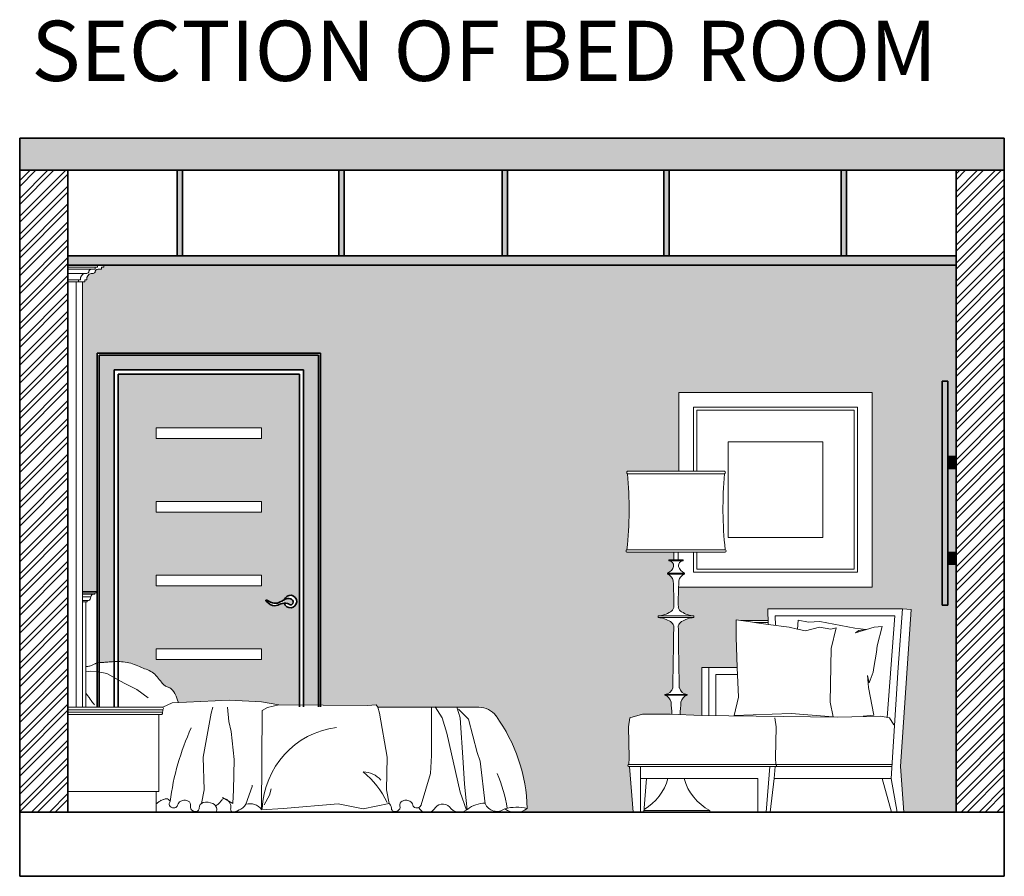
# Model space of a CAD drawing. Units: inches. Extents: x 64 to 1167, y 117 to 939.
# Tile 28 of 56: x 592 to 776, y 435 to 596. Entities that reach past the tile are written whole.
import ezdxf

# ---------------------------------------------------------------- set-up
doc = ezdxf.new("R2010")
doc.units = ezdxf.units.IN
doc.header["$MEASUREMENT"] = 0
for name, color, linetype, lineweight in [('A-ANNO-TEXT', 7, 'Continuous', 25), ('A-FURN', 8, 'Continuous', 18), ('A-SECT', 7, 'Continuous', 35), ('A-SECT-DETL', 8, 'Continuous', 18), ('A-SECT-PATT', 252, 'Continuous', 13)]:
    doc.layers.add(name, color=color, linetype=linetype, lineweight=lineweight)
doc.styles.get("Standard").update_dxf_attribs({"font": 'arial.ttf'})
pattern_1 = [(45, (-379.0635, 744.1152), (-1.67054, 1.67054), []), (45, (-377.9498, 744.1152), (-1.67054, 1.67054), [])]

# ---------------------------------------------------------------- blocks, each defined once
blk = doc.blocks.new('A$C19551A3F')
at = {"ltscale": 0.75}
for p, q in [((46.01, 78.48), (9.85, 78.48)), ((9.85, 78.48), (9.85, 63.74)), ((46.01, 42.09), (46.01, 78.48)), ((0.27, 63.74), (18.4, 63.74)), ((8.91, 48.6), (0.15, 48.6)), ((8.91, 48.6), (8.91, 47.17)), ((9.77, 48.6), (18.53, 48.6)), ((9.77, 48.6), (9.77, 47.17)), ((7.98, 47.17), (8.91, 47.17)), ((7.98, 47.17), (7.98, 47.01)), ((10.7, 47.17), (9.77, 47.17)), ((10.7, 47.17), (10.7, 47.01)), ((7.75, 44.52), (7.75, 44.68)), ((10.93, 44.52), (10.93, 44.68)), ((9.81, 42.09), (46.01, 42.09)), ((51.65, 38.02), (26.5, 38.02)), ((26.5, 38.02), (26.58, 35.09)), ((51.29, 8.52), (53.27, 37.86)), ((51.65, 38.02), (53.27, 37.86)), ((5.99, 36.69), (5.99, 36.39)), ((12.69, 36.69), (12.69, 36.39)), ((20.55, 32.71), (20.55, 35.96)), ((20.55, 35.96), (23.26, 35.55)), ((23.26, 35.55), (24.38, 35.38)), ((24.38, 35.38), (26.58, 35.09)), ((20.79, 27.02), (20.55, 32.71)), ((14.18, 18.04), (14.18, 27.02)), ((20.79, 27.02), (14.18, 27.02)), ((7.27, 21.84), (7.27, 22)), ((11.4, 21.84), (11.4, 22)), ((0.71, 17.65), (0.43, 15.95)), ((3.06, 18.32), (0.71, 17.65)), ((8.24, 18.32), (3.06, 18.32)), ((14.18, 18.04), (8.24, 18.32)), ((0.43, 15.95), (0.57, 10.15)), ((0.57, 10.15), (0.51, 8.93)), ((0.35, 8.68), (0.4, 8.93)), ((0.51, 8.51), (0.35, 8.68)), ((0.4, 8.93), (0.51, 8.93)), ((0.65, 8.51), (0.51, 8.51)), ((0.65, 8.51), (1.33, 0)), ((51.29, 8.52), (51.9, 0)), ((3.85, 6.28), (3.35, 0)), ((7.66, 6.28), (3.85, 6.28)), ((24.65, 6.28), (7.66, 6.28)), ((24.65, 6.28), (24.64, 0)), ((27.67, 6.28), (26.93, 0)), ((47.84, 6.28), (27.67, 6.28)), ((49.58, 0), (47.84, 6.28)), ((15.64, 0.32), (15.64, 0))]:
    blk.add_line(p, q, dxfattribs=at)
for p, q in [((43.25, 75.72), (12.61, 75.72)), ((12.61, 75.72), (12.61, 63.74)), ((43.25, 44.84), (43.25, 75.72)), ((42.66, 75.13), (13.2, 75.13)), ((13.2, 75.13), (13.2, 63.74)), ((42.66, 45.43), (42.66, 75.13)), ((36.75, 69.22), (19.11, 69.22)), ((19.11, 69.22), (19.11, 51.34)), ((36.75, 51.34), (36.75, 69.22)), ((18.4, 63.27), (0.27, 63.27)), ((19.11, 51.34), (36.75, 51.34)), ((0.15, 49.07), (18.53, 49.07)), ((9.77, 48.6), (8.91, 48.6)), ((12.61, 48.6), (12.61, 44.84)), ((13.2, 48.6), (13.2, 45.43)), ((7.98, 47.01), (9.34, 47.01)), ((9.77, 47.17), (8.91, 47.17)), ((10.7, 47.01), (9.34, 47.01)), ((7.75, 44.68), (9.34, 44.68)), ((7.75, 44.52), (9.34, 44.52)), ((10.93, 44.68), (9.34, 44.68)), ((10.93, 44.52), (9.34, 44.52)), ((12.61, 44.84), (43.25, 44.84)), ((13.2, 45.43), (42.66, 45.43)), ((50.84, 27.02), (51.65, 38.02)), ((5.99, 36.69), (9.34, 36.69)), ((5.99, 36.39), (9.34, 36.39)), ((12.69, 36.69), (9.34, 36.69)), ((12.69, 36.39), (9.34, 36.39)), ((21.47, 35.82), (26.56, 35.82)), ((24.06, 35.43), (26.58, 35.43)), ((26.58, 35.09), (30.51, 34.57)), ((50.2, 36.68), (27.89, 36.68)), ((27.89, 36.68), (27.94, 34.91)), ((32.17, 35.87), (32.01, 34.22)), ((34.12, 35.49), (32.17, 35.87)), ((36.21, 35.61), (34.12, 35.49)), ((42.74, 34.39), (36.21, 35.61)), ((48.81, 17.69), (50.2, 36.68)), ((30.51, 34.57), (32.02, 34.22)), ((32.02, 34.22), (33.53, 33.87)), ((33.53, 33.87), (36.15, 34.57)), ((36.15, 34.57), (38.24, 34.22)), ((38.24, 34.22), (39.29, 34.45)), ((39.29, 34.45), (38.36, 30.61)), ((44.9, 34.13), (42.74, 34.39)), ((46.34, 34.57), (42.85, 33.52)), ((42.85, 33.52), (43.49, 33.98)), ((43.49, 33.98), (44.9, 34.13)), ((47.85, 34.68), (46.34, 34.57)), ((46.92, 31.08), (47.85, 34.68)), ((38.36, 30.61), (38.13, 20.54)), ((46.81, 29.93), (46.3, 27.02)), ((46.81, 29.93), (46.92, 31.08)), ((15.44, 27.02), (15.44, 18.03)), ((21.02, 21.47), (20.79, 27.02)), ((46.15, 26.14), (45.42, 24.16)), ((46.3, 27.02), (46.15, 26.14)), ((49.55, 6.28), (50.84, 27.02)), ((16.76, 18.02), (16.76, 25.75)), ((20.84, 25.75), (16.76, 25.75)), ((45.42, 24.16), (45.11, 25.52)), ((45.11, 25.52), (45.32, 23.33)), ((45.32, 23.33), (46.3, 18.11)), ((7.27, 22), (9.34, 22)), ((7.27, 21.84), (9.34, 21.84)), ((11.4, 22), (9.34, 22)), ((11.4, 21.84), (9.34, 21.84)), ((20.23, 18.06), (21.02, 21.47)), ((38.13, 20.54), (38.71, 17.83)), ((30.86, 18.44), (20.23, 18.06)), ((38.71, 17.83), (30.86, 18.44)), ((39.52, 17.75), (14.18, 18.04)), ((27.79, 17.65), (28.06, 15.95)), ((47.59, 17.92), (39.52, 17.75)), ((46.3, 18.11), (44.28, 17.92)), ((49.25, 17.61), (47.59, 17.92)), ((50.06, 16.35), (49.25, 17.61)), ((28.06, 15.95), (27.93, 10.15)), ((27.93, 10.15), (27.99, 8.93)), ((7.79, 8.93), (0.51, 8.93)), ((7.77, 8.51), (0.65, 8.51)), ((2.72, 6.28), (2.72, 8.51)), ((49.63, 8.51), (7.77, 8.51)), ((49.63, 8.93), (7.79, 8.93)), ((26.89, 8.51), (26.18, 0)), ((27.85, 8.51), (27.67, 6.28)), ((27.85, 8.51), (27.99, 8.51)), ((28.1, 8.93), (27.99, 8.93)), ((27.99, 8.51), (28.14, 8.68)), ((28.14, 8.68), (28.1, 8.93)), ((2.72, 6.28), (2.72, 0)), ((3.85, 6.28), (2.72, 6.28)), ((47.84, 6.28), (49.55, 6.28)), ((50.69, 0), (49.55, 6.28)), ((15.64, 0.32), (3.37, 0.32)), ((1.33, 0), (15.64, 0)), ((24.64, 0), (26.93, 0)), ((49.58, 0), (51.9, 0))]:
    blk.add_line(p, q)
for centre, radius, start, end in [((0.38, 63.5), 0.259, 114.7637, 245.2363), ((-71.6, 56.79), 72.17, 353.8588, 5.1523), ((90.28, 56.79), 72.17, 174.8477, 186.1412), ((18.3, 63.5), 0.259, 294.7637, 65.2363), ((0.26, 48.83), 0.259, 114.7637, 245.2363), ((18.42, 48.83), 0.259, 294.7637, 65.2363), ((7.93, 46.06), 0.958, 353.355, 87.0766), ((10.75, 46.06), 0.958, 92.9234, 186.645), ((7.01, 46.49), 1.95, 292.4844, 343.8815), ((7.01, 42.82), 1.86, 13.8227, 66.4869), ((11.67, 46.49), 1.95, 196.1185, 247.5156), ((11.67, 42.82), 1.86, 113.5131, 166.1773), ((-52.9, 39.63), 61.82, 358.7223, 3.3675), ((71.58, 39.63), 61.82, 176.6325, 181.2777), ((5.72, 41.37), 4.68, 273.314, 303.4025), ((7.73, 38.52), 1.21, 298.1279, 347.3635), ((10.95, 38.52), 1.21, 192.6365, 241.8721), ((12.96, 41.37), 4.68, 236.5975, 266.686), ((5.72, 31.71), 4.68, 56.5975, 86.686), ((7.73, 34.56), 1.21, 12.6365, 61.8721), ((10.95, 34.56), 1.21, 118.1279, 167.3635), ((12.96, 31.71), 4.68, 93.314, 123.4025), ((-1024.36, 45.37), 1033.32, 358.7741, 359.41551), ((1043.03, 45.37), 1033.32, 180.58449, 181.2259), ((7.11, 23.65), 1.66, 275.7149, 346.2729), ((11.57, 23.65), 1.66, 193.7271, 264.2851), ((6.79, 20.26), 1.65, 11.2443, 73.1809), ((-51.51, 15.45), 60.14, 2.7194, 4.8893), ((70.18, 15.45), 60.14, 175.1107, 177.3513), ((11.88, 20.26), 1.65, 106.8191, 168.7557), ((-1.63, 8.99), 9.85, 300.6248, 343.9923), ((20.31, 8.99), 9.85, 196.0077, 241.7222)]:
    blk.add_arc(centre, radius, start, end, dxfattribs=at)
blk = doc.blocks.new('A$C09710878')
for p, q in [((0, 102.38), (0, 0.02)), ((5.12, 101.99), (0, 101.99)), ((4.56, 101.61), (0, 101.61)), ((1.18, 102.38), (6.69, 102.38)), ((6.3, 101.59), (5.91, 101.59)), ((6.69, 101.99), (6.3, 101.99)), ((6.3, 101.99), (6.3, 101.59)), ((6.69, 102.38), (6.69, 101.99)), ((3.54, 100.81), (0, 100.81)), ((1.97, 99.63), (0, 99.63)), ((3.54, 99.63), (3.15, 99.63)), ((3.15, 99.63), (3.15, 99.23)), ((3.54, 100.02), (3.54, 99.63)), ((3.15, 99.23), (1.18, 99.23)), ((2.76, 99.23), (2.76, 19.7)), ((2.76, 41.36), (5.26, 41.36)), ((5.02, 41.11), (2.76, 41.11)), ((4.95, 40.87), (2.76, 40.87)), ((5.02, 40.87), (4.95, 40.87)), ((5.26, 41.11), (5.02, 41.11)), ((5.02, 41.11), (5.02, 40.87)), ((5.26, 41.36), (5.26, 41.11)), ((4.27, 40.32), (2.76, 40.32)), ((3.59, 39.64), (2.76, 39.64)), ((3.59, 39.39), (2.76, 39.39)), ((3.35, 39.39), (3.35, 19.7)), ((3.84, 39.64), (3.59, 39.64)), ((3.59, 39.64), (3.59, 39.39)), ((4.65, 27.61), (4.51, 27.55)), ((4.8, 27.67), (4.65, 27.61)), ((4.93, 27.74), (4.8, 27.67)), ((5.07, 27.8), (4.93, 27.74)), ((5.19, 27.86), (5.07, 27.8)), ((5.31, 27.91), (5.19, 27.86)), ((5.43, 27.96), (5.31, 27.91)), ((5.53, 28), (5.43, 27.96)), ((5.63, 28.02), (5.53, 28)), ((5.73, 28.04), (5.63, 28.02)), ((5.83, 28.05), (5.73, 28.04)), ((5.93, 28.06), (5.83, 28.05)), ((6.05, 28.06), (5.93, 28.06)), ((6.18, 28.06), (6.05, 28.06)), ((6.33, 28.06), (6.18, 28.06)), ((6.5, 28.07), (6.33, 28.06)), ((6.7, 28.09), (6.5, 28.07)), ((6.93, 28.11), (6.7, 28.09)), ((7.18, 28.13), (6.93, 28.11)), ((7.45, 28.15), (7.18, 28.13)), ((7.74, 28.17), (7.45, 28.15)), ((8.04, 28.2), (7.74, 28.17)), ((8.35, 28.22), (8.04, 28.2)), ((8.67, 28.23), (8.35, 28.22)), ((9, 28.24), (8.67, 28.23)), ((9.34, 28.24), (9, 28.24)), ((9.68, 28.23), (9.34, 28.24)), ((10.02, 28.22), (9.68, 28.23)), ((10.36, 28.18), (10.02, 28.22)), ((10.71, 28.14), (10.36, 28.18)), ((11.05, 28.08), (10.71, 28.14)), ((11.4, 28.01), (11.05, 28.08)), ((11.74, 27.92), (11.4, 28.01)), ((12.08, 27.81), (11.74, 27.92)), ((12.42, 27.69), (12.08, 27.81)), ((12.75, 27.56), (12.42, 27.69)), ((3.44, 27.29), (3.29, 27.29)), ((4.23, 26.46), (3.36, 26.35)), ((3.59, 27.31), (3.44, 27.29)), ((3.74, 27.33), (3.59, 27.31)), ((3.9, 27.36), (3.74, 27.33)), ((4.05, 27.4), (3.9, 27.36)), ((4.21, 27.44), (4.05, 27.4)), ((4.36, 27.49), (4.21, 27.44)), ((5.69, 26.29), (4.23, 26.46)), ((4.51, 27.55), (4.36, 27.49)), ((7.26, 26), (5.69, 26.29)), ((10.52, 24.19), (7.26, 26)), ((13.08, 27.43), (12.75, 27.56)), ((13.41, 27.3), (13.08, 27.43)), ((13.73, 27.16), (13.41, 27.3)), ((14.04, 27.03), (13.73, 27.16)), ((14.34, 26.91), (14.04, 27.03)), ((14.64, 26.79), (14.34, 26.91)), ((14.93, 26.67), (14.64, 26.79)), ((15.21, 26.54), (14.93, 26.67)), ((15.48, 26.4), (15.21, 26.54)), ((15.74, 26.24), (15.48, 26.4)), ((15.99, 26.07), (15.74, 26.24)), ((16.23, 25.87), (15.99, 26.07)), ((16.46, 25.64), (16.23, 25.87)), ((12.91, 23.03), (10.52, 24.19)), ((16.68, 25.4), (16.46, 25.64)), ((16.89, 25.14), (16.68, 25.4)), ((17.09, 24.88), (16.89, 25.14)), ((17.28, 24.63), (17.09, 24.88)), ((17.47, 24.39), (17.28, 24.63)), ((17.64, 24.18), (17.47, 24.39)), ((17.81, 24), (17.64, 24.18)), ((17.97, 23.85), (17.81, 24)), ((3.34, 22.36), (3.69, 21.88)), ((15.01, 21.45), (12.91, 23.03)), ((18.12, 23.74), (17.97, 23.85)), ((18.27, 23.66), (18.12, 23.74)), ((18.42, 23.59), (18.27, 23.66)), ((18.57, 23.53), (18.42, 23.59)), ((18.72, 23.47), (18.57, 23.53)), ((18.88, 23.4), (18.72, 23.47)), ((19.04, 23.32), (18.88, 23.4)), ((19.21, 23.22), (19.04, 23.32)), ((19.39, 23.07), (19.21, 23.22)), ((19.58, 22.87), (19.39, 23.07)), ((19.78, 22.61), (19.58, 22.87)), ((19.99, 22.25), (19.78, 22.61)), ((20.21, 21.79), (19.99, 22.25)), ((3.69, 21.88), (3.96, 21.51)), ((3.96, 21.51), (4.17, 21.22)), ((4.17, 21.22), (4.34, 20.99)), ((4.34, 20.99), (4.48, 20.79)), ((4.48, 20.79), (4.63, 20.6)), ((4.63, 20.6), (4.8, 20.39)), ((4.8, 20.39), (5, 20.13)), ((19.52, 20.54), (17.72, 19.7)), ((30.18, 21.04), (19.52, 20.54)), ((20.45, 21.21), (20.21, 21.79)), ((20.69, 20.5), (20.45, 21.21)), ((36.19, 20.71), (30.18, 21.04)), ((39.41, 20.16), (36.19, 20.71)), ((17.72, 19.7), (0, 19.7)), ((17.72, 19.23), (0, 19.23)), ((17.66, 18.8), (0, 18.8)), ((25.3, 10.36), (26.75, 18.62)), ((26.75, 18.62), (27.06, 19.7)), ((30.08, 17.02), (29.83, 19.7)), ((36.34, 19.09), (36.21, 0.55)), ((37.31, 19.68), (36.34, 19.09)), ((39.41, 20.16), (37.31, 19.68)), ((55.99, 20), (39.41, 20.16)), ((57.61, 20.14), (55.99, 20)), ((57.92, 19.7), (57.61, 20.14)), ((57.92, 19.7), (76.81, 19.7)), ((58.23, 18.62), (57.92, 19.7)), ((59.68, 10.36), (58.23, 18.62)), ((67.94, 14.56), (67.94, 19.7)), ((69.94, 17.75), (68.64, 19.78)), ((73.28, 17.75), (72.68, 19.7)), ((72.99, 19.34), (74.87, 17.46)), ((17.59, 18.33), (0, 18.33)), ((17, 18.33), (17, 3.96)), ((30.52, 15.14), (30.08, 17.02)), ((70.81, 14.85), (69.94, 17.75)), ((73.86, 9.35), (73.28, 17.75)), ((74.87, 17.46), (76.47, 11.23)), ((31.1, 9.93), (30.52, 15.14)), ((73.28, 3.85), (70.81, 14.85)), ((67.94, 10.65), (67.94, 14.56)), ((76.47, 11.23), (77.05, 9.64)), ((25.44, 4.28), (25.3, 10.36)), ((30.95, 4.28), (31.1, 9.93)), ((59.53, 4.28), (59.68, 10.36)), ((67.79, 7.32), (67.94, 10.65)), ((74.15, 5.3), (73.86, 9.35)), ((77.05, 9.64), (78, 1.66)), ((66.04, 1.43), (67.79, 7.32)), ((17, 3.96), (0, 3.96)), ((16.53, 3.96), (16.53, 0.02)), ((24.96, 1.72), (25.44, 4.28)), ((30.81, 1.68), (30.95, 4.28)), ((33.26, 1.56), (34.42, 4.89)), ((34.42, 4.89), (34.45, 5.12)), ((37.97, 4.47), (37.65, 3.27)), ((60.02, 1.72), (59.53, 4.28)), ((74.51, 0.48), (73.28, 3.85)), ((74.44, 2.26), (74.15, 5.3)), ((28.92, 2.84), (30.81, 1.68)), ((37.65, 3.27), (36.68, 1.45)), ((74.59, 0.54), (74.44, 2.26)), ((0, 0.02), (83.76, 0.02)), ((36.21, 0.55), (40.22, 0.76)), ((40.22, 0.76), (50.5, 1.64)), ((50.5, 1.64), (55.18, 0.7)), ((55.18, 0.7), (60.02, 1.72))]:
    blk.add_line(p, q)
at = {"ltscale": 150}
for p, q in [((0, 102.38), (5.51, 102.38)), ((5.12, 101.59), (4.72, 101.59)), ((5.51, 101.99), (5.12, 101.99)), ((5.12, 101.99), (5.12, 101.59)), ((5.51, 102.38), (5.51, 101.99)), ((2.36, 99.63), (1.97, 99.63)), ((1.97, 99.63), (1.97, 99.23)), ((2.36, 100.02), (2.36, 99.63)), ((1.97, 99.23), (0, 99.23)), ((1.57, 99.23), (1.57, 19.7))]:
    blk.add_line(p, q, dxfattribs=at)
for centre, radius, start, end in [((3.54, 101.2), 0.394, 270, 0), ((4.56, 100.94), 0.678, 76.1085, 157.0216), ((3.39, 99.76), 1.06, 81.4808, 165.8993)]:
    blk.add_arc(centre, radius, start, end, dxfattribs=at)
for centre, radius, start, end in [((4.72, 101.2), 0.394, 270, 0), ((5.74, 100.94), 0.678, 76.1085, 157.0216), ((4.57, 99.76), 1.06, 81.4808, 165.8993), ((4.92, 40.21), 0.66, 87.4212, 169.929), ((3.54, 40.3), 0.73, 293.7928, 1.5008), ((17.15, 18.63), 0.536, 324.9774, 17.9545), ((17.45, 19.04), 0.326, 310.9941, 35.0512), ((17.61, 19.47), 0.26, 294.6112, 65.3888), ((76.81, 15.77), 3.94, 35.832, 90), ((54.99, 0.01), 30.86, 1.457, 35.832), ((68.32, -4.61), 49.68, 155.6902, 172.2902), ((52.27, 0.14), 15.94, 97.5724, 178.0202), ((44.32, -5.48), 17.03, 25.5693, 50.2938), ((55.12, 3.19), 4.43, 40.7088, 88.9264), ((57.05, -2.86), 25.31, 8.3744, 23.7338), ((10.23, 9.8), 10.31, 307.6312, 310.5669), ((18.82, -0.51), 3.12, 115.9381, 127.154), ((20.37, -3.7), 6.65, 111.7814, 115.9381), ((18.68, 0.53), 2.1, 104.378, 111.7814), ((18.35, 1.82), 0.769, 71.5824, 104.378), ((18.29, 1.65), 0.954, 42.229, 71.5824), ((18.73, 2.05), 0.363, 320.3102, 42.229), ((21.51, 1.23), 1.01, 114.2927, 169.7827), ((21.83, 0.53), 1.78, 90, 114.2927), ((21.83, 0.82), 1.49, 63.4272, 90), ((22.13, 1.43), 0.801, 346.0902, 63.4272), ((25.55, 0.88), 1.02, 104.5937, 181.7578), ((25.94, -0.61), 2.57, 63.4581, 104.5937), ((22.67, 7.51), 8.02, 314.9709, 315.949), ((27.43, 2.91), 1.4, 315.949, 329.8173), ((30.02, 1.4), 1.59, 136.799, 149.8173), ((29.17, 2.2), 0.428, 81.878, 136.799), ((29.06, 1.42), 1.21, 50.0773, 81.878), ((28.96, 1.3), 1.37, 33.7168, 50.0773), ((27.17, 0.11), 3.52, 23.5428, 33.7168), ((62.84, 1.43), 0.801, 116.5728, 193.9098), ((63.15, 0.82), 1.49, 90, 116.5728), ((63.15, 0.53), 1.78, 65.7073, 90), ((63.47, 1.23), 1.01, 10.2173, 65.7073), ((19.32, 1.56), 0.403, 140.3102, 217.2793), ((20.22, 2.24), 1.54, 217.2793, 233.1579), ((19.71, 1.56), 0.69, 233.1579, 256.9409), ((19.71, 1.55), 0.677, 256.9409, 270), ((19.71, 2.91), 2.04, 270, 277.5153), ((19.89, 1.52), 0.631, 277.5153, 349.7827), ((23.69, 1.05), 0.798, 166.0902, 243.5813), ((24, 1.68), 1.51, 243.5813, 251.5824), ((24.11, 2.01), 1.85, 251.5824, 258.8111), ((23.88, 0.83), 0.649, 258.8111, 1.7578), ((26.5, 0.51), 1.32, 4.6698, 63.4581), ((26.54, 3.3), 2.31, 296.8941, 314.4523), ((28.08, 0.29), 0.291, 170.6484, 198.6345), ((26.67, 0.52), 1.14, 350.6484, 4.6698), ((28.02, 0.26), 0.22, 198.6345, 218.4296), ((8.17, 22.03), 28.54, 314.4523, 314.9709), ((29.43, 1.1), 1.05, 343.6974, 23.5428), ((31.04, 0.63), 0.626, 163.6974, 216.058), ((30.86, 0.49), 0.402, 216.058, 282.9819), ((29.9, 4.68), 4.7, 282.9819, 301.5385), ((30.83, 3.15), 2.91, 301.5385, 318.3377), ((30.82, 3.17), 2.93, 318.3377, 326.7067), ((34.01, -1.06), 2.73, 36.6754, 105.7915), ((37.7, 2.24), 2.26, 227.995, 228.6577), ((59.43, 0.88), 1.02, 358.2422, 61.1681), ((61.1, 0.83), 0.649, 178.2422, 281.1889), ((60.87, 2.01), 1.85, 281.1889, 288.4176), ((60.97, 1.68), 1.51, 288.4176, 296.4187), ((61.29, 1.05), 0.798, 296.4187, 13.9098), ((65.08, 1.52), 0.631, 190.2173, 262.4847), ((65.27, 2.91), 2.04, 262.4847, 270), ((65.27, 1.55), 0.677, 270, 283.0591), ((65.26, 1.56), 0.69, 283.0591, 306.8421), ((67.11, 1.71), 1.71, 208.0597, 320.5306), ((64.76, 2.24), 1.54, 306.8421, 322.7207), ((65.66, 1.56), 0.403, 322.7207, 344.9141), ((70.06, -0.25), 1.85, 46.7208, 151.7813), ((73.22, 2.33), 2.26, 213.2377, 312.005), ((78.09, -3.74), 5.53, 91.3545, 127.5096), ((80.19, 2.58), 2.36, 201.7886, 308.3305), ((83.89, -7.65), 8.66, 77.0554, 104.9473), ((83.7, 3.34), 3.32, 232.0778, 309.9248)]:
    blk.add_arc(centre, radius, start, end)
blk = doc.blocks.new('DOOR-PANEL-GROOVE')
for p, q in [((19.69, 1.97), (0, 1.97)), ((0, 1.97), (0, 0)), ((19.69, 0), (19.69, 1.97)), ((0, 0), (19.69, 0))]:
    blk.add_line(p, q)

msp = doc.modelspace()

# ---------------------------------------------------------------- hatches: boundary and pattern name
at = {"layer": 'A-SECT-PATT'}
h = msp.add_hatch(dxfattribs=at)
h.set_pattern_fill('AR-CONC', color=256, scale=0.89)
h.set_pattern_definition([(50, (-379.0635, 744.115), (6.383616, -0.558494), [0.6675, -7.3425]), (355, (-379.0635, 744.115), (-1.234887, 6.69451), [0.534, -5.874]), (100.45144, (-378.5315, 744.0687), (5.14873, 6.136016), [0.567288, -6.240165]), (46.1842, (-379.0635, 745.895), (9.49845, -1.47312), [1.00125, -11.01375]), (96.6356, (-378.272, 745.772), (8.31849, 8.669656), [0.85093, -9.36025]), (351.1842, (-379.063, 745.895), (8.31849, 8.669656), [0.801, -8.811]), (21, (-378.1735, 745.45), (5.312473, -3.583308), [0.6675, -7.3425]), (326, (-378.1735, 745.45), (2.165506, 6.453835), [0.534, -5.874]), (71.45144, (-377.731, 745.1516), (7.47798, 2.870527), [0.567288, -6.240165]), (37.5, (-379.0635, 744.1152), (0.1082227, 2.9627553), [0, -5.8028, 0, -5.963, 0, -5.89625]), (7.5, (-379.0635, 744.1152), (2.341319, 3.510264), [0, -3.3998, 0, -5.6693, 0, -2.24725]), (327.5, (-381.0482, 744.1152), (4.7510197, -0.2007384), [0, -2.225, 0, -6.942, 0, -9.2115]), (317.5, (-381.938, 744.115), (5.190357, 0.890934), [0, -2.8925, 0, -4.6102, 0, -6.5415])])
h.paths.add_polyline_path([(775.58, 567.35), (775.58, 573.35), (591.58, 573.35), (591.58, 567.35)])
h = msp.add_hatch(dxfattribs=at)
h.set_pattern_fill('ANSI32', color=256, scale=6.3)
h.set_pattern_definition(pattern_1)
h.paths.add_polyline_path([(591.58, 447.35), (600.58, 447.35), (600.58, 549.64), (600.58, 567.35), (591.58, 567.35)])
h = msp.add_hatch(color=256, dxfattribs=at)
h.dxf.hatch_style = 1
h.paths.add_polyline_path([(622.01, 567.35), (621.01, 567.35), (621.01, 551.35), (622.01, 551.35)])
h = msp.add_hatch(color=256, dxfattribs=at)
h.dxf.hatch_style = 1
h.paths.add_polyline_path([(652.24, 567.35), (651.24, 567.35), (651.24, 551.35), (652.24, 551.35)])
h = msp.add_hatch(color=256, dxfattribs=at)
h.dxf.hatch_style = 1
h.paths.add_polyline_path([(681.71, 551.35), (682.71, 551.35), (682.71, 567.35), (681.71, 567.35)])
h = msp.add_hatch(color=256, dxfattribs=at)
h.dxf.hatch_style = 1
h.paths.add_polyline_path([(711.94, 551.35), (712.94, 551.35), (712.94, 567.35), (711.94, 567.35)])
h = msp.add_hatch(color=256, dxfattribs=at)
h.dxf.hatch_style = 1
h.paths.add_polyline_path([(745.1, 551.35), (746.1, 551.35), (746.1, 567.35), (745.1, 567.35)])
h = msp.add_hatch(dxfattribs=at)
h.set_pattern_fill('ANSI32', color=256, scale=6.3)
h.set_pattern_definition(pattern_1)
h.paths.add_polyline_path([(766.58, 447.35), (775.58, 447.35), (775.58, 567.35), (766.58, 567.35)])
h = msp.add_hatch(color=256, dxfattribs=at)
h.dxf.hatch_style = 1
h.paths.add_polyline_path([(766.58, 551.35), (600.58, 551.35), (600.58, 549.64), (766.58, 549.64)])
h = msp.add_hatch(color=256, dxfattribs=at)
h.dxf.hatch_style = 1
h.paths.add_polyline_path([(766.58, 549.64), (607.27, 549.64), (607.27, 549.25), (606.88, 549.25), (606.88, 548.85), (606.48, 548.85, 0.368489), (605.69, 548.46, -0.479218), (605.22, 548.07, 0.362974), (604.12, 547.28), (604.12, 546.88), (603.73, 546.88), (603.73, 546.49), (603.33, 546.49), (603.33, 488.62), (606.06, 488.62), (606.06, 533.18), (647.79, 533.18), (647.79, 467.34), (656.57, 467.26), (658.18, 467.4), (658.5, 466.96), (677.39, 466.96, -0.240854), (680.58, 465.33, -0.151124), (686.41, 448.05, -0.122293), (684.97, 447.35), (706.22, 447.35), (705.54, 455.86), (705.4, 455.86), (705.24, 456.03), (705.29, 456.28), (705.4, 456.28), (705.46, 457.5), (705.33, 463.3), (705.6, 465), (707.95, 465.67), (713.14, 465.67), (713.46, 465.66, 0.009469), (713.31, 467.93, 0.277027), (712.17, 469.19), (712.17, 469.35, 0.317978), (713.61, 470.61, 0.002799), (713.8, 482.17, 0.154066), (713.43, 482.8, 0.148296), (710.88, 483.74), (710.88, 484.04, 0.148296), (713.43, 484.98, 0.154066), (713.8, 485.6, 0.020271), (713.71, 490.61, 0.268611), (712.42, 491.96, 0.260891), (713.77, 493.29, 0.464017), (712.77, 494.36), (712.87, 494.36), (712.87, 494.52), (713.8, 494.52), (713.8, 495.95), (705.26, 495.95, -1), (705.04, 496.42, 0.049317), (705.17, 510.62, -0.639973), (705.17, 511.09), (714.75, 511.09), (714.75, 525.82), (750.9, 525.82), (750.9, 489.44), (714.7, 489.44, 0.0155), (714.66, 485.6, 0.154066), (715.03, 484.98, 0.148296), (717.58, 484.04), (717.58, 483.74, 0.148296), (715.03, 482.8, 0.154066), (714.66, 482.17, 0.002799), (714.85, 470.61, 0.317978), (716.3, 469.35), (716.3, 469.19, 0.277027), (715.15, 467.93, 0.009777), (715, 465.58), (719.08, 465.39), (719.08, 474.37), (725.68, 474.37), (725.45, 480.06), (725.45, 483.31), (726.36, 483.17), (731.46, 483.17), (731.4, 485.37), (756.54, 485.37), (758.16, 485.21), (756.18, 455.87), (756.79, 447.35), (766.58, 447.35), (766.58, 493.7), (765, 493.7), (765, 486.06), (763.99, 486.06), (763.99, 527.94), (765, 527.94), (765, 513.81), (766.58, 513.81)])
h = msp.add_hatch(color=256, dxfattribs=at)
h.dxf.hatch_style = 1
h.paths.add_polyline_path([(647.4, 532.78), (606.45, 532.78), (606.45, 475.31), (607.52, 475.36), (609.21, 475.51), (609.21, 530.03), (644.64, 530.03), (644.64, 467.38), (647.4, 467.35)])
h = msp.add_hatch(color=256, dxfattribs=at)
h.dxf.hatch_style = 1
h.paths.add_polyline_path([(643.86, 529.24), (610, 529.24), (610, 475.56), (612.07, 475.3), (614.62, 474.33), (616.65, 473.39), (618.47, 471.18), (618.55, 471.11), (620.19, 470.3), (621.36, 467.86), (630.76, 468.3), (636.77, 467.97), (639.99, 467.42), (643.86, 467.38)])
h.paths.add_polyline_path([(636.77, 517.23), (617.08, 517.23), (617.08, 519.2), (636.77, 519.2)], flags=16)
h.paths.add_polyline_path([(617.08, 503.45), (617.08, 505.42), (636.77, 505.42), (636.77, 503.45)], flags=16)
h.paths.add_polyline_path([(617.08, 489.67), (617.08, 491.64), (636.77, 491.64), (636.77, 489.67)], flags=16)
edge = h.paths.add_edge_path(flags=16)
edge.add_spline(control_points=[(637.63, 486.8), (637.61, 486.87), (637.54, 487.1), (638.54, 486.52), (639.28, 486.24), (640.69, 486.77), (641.64, 487.54), (642.92, 486.96), (642.39, 485.83), (641.68, 486.44), (641.21, 486.47), (641.01, 486.45)], knot_values=[3.655363, 3.655363, 3.655363, 3.655363, 3.838213, 4.244746, 5.790106, 6.948902, 8.393382, 9.32042, 10.047955, 10.84947, 11.433768, 11.433768, 11.433768, 11.433768], degree=3, periodic=0)
edge.add_arc((642.16, 486.72), 1.18, -166.7121, 176.8362, ccw=False)
edge.add_spline(control_points=[(641.01, 486.45), (640.39, 486.37), (639.19, 485.48), (638.15, 486.36), (637.63, 486.8)], knot_values=[0, 0, 0, 0, 1.841528, 3.655363, 3.655363, 3.655363, 3.655363], degree=3, periodic=0)
h.paths.add_polyline_path([(617.08, 475.89), (617.08, 477.86), (636.77, 477.86), (636.77, 475.89)], flags=16)
h = msp.add_hatch(color=256, dxfattribs=at)
h.dxf.hatch_style = 1
h.paths.add_polyline_path([(765, 527.94), (763.99, 527.94), (763.99, 486.06), (765, 486.06)])
h = msp.add_hatch(color=256, dxfattribs=at)
h.dxf.hatch_style = 1
h.paths.add_polyline_path([(766.58, 513.81), (765, 513.81), (765, 511.59), (766.58, 511.59)])
h = msp.add_hatch(color=256, dxfattribs=at)
h.dxf.hatch_style = 1
h.paths.add_polyline_path([(766.58, 511.59), (765, 511.59), (765, 495.92), (766.58, 495.92)])
h = msp.add_hatch(color=256, dxfattribs=at)
h.dxf.hatch_style = 1
h.paths.add_polyline_path([(766.58, 495.92), (765, 495.92), (765, 493.7), (766.58, 493.7)])

# ---------------------------------------------------------------- linework, layer by layer
at = {"layer": 'A-SECT'}
for p, q in [((591.58, 435.35), (591.58, 573.35)), ((775.58, 573.35), (591.58, 573.35)), ((775.58, 573.35), (775.58, 435.35)), ((775.58, 567.35), (591.58, 567.35)), ((600.58, 447.35), (600.58, 567.35)), ((621.01, 567.35), (621.01, 551.35)), ((622.01, 567.35), (622.01, 551.35)), ((651.24, 567.35), (651.24, 551.35)), ((652.24, 567.35), (652.24, 551.35)), ((681.71, 567.35), (681.71, 551.35)), ((682.71, 567.35), (682.71, 551.35)), ((711.94, 567.35), (711.94, 551.35)), ((712.94, 567.35), (712.94, 551.35)), ((745.1, 567.35), (745.1, 551.35)), ((746.1, 567.35), (746.1, 551.35)), ((766.58, 567.35), (766.58, 447.35)), ((600.58, 551.35), (766.58, 551.35)), ((600.58, 549.64), (766.58, 549.64)), ((606.06, 467.06), (606.06, 533.18)), ((606.06, 533.18), (647.79, 533.18)), ((606.45, 467.06), (606.45, 532.78)), ((606.45, 532.78), (647.4, 532.78)), ((647.4, 532.78), (647.4, 467.06)), ((647.79, 533.18), (647.79, 467.06)), ((609.21, 530.03), (609.21, 467.06)), ((644.64, 530.03), (609.21, 530.03)), ((644.64, 467.06), (644.64, 530.03)), ((610, 529.24), (610, 467.06)), ((643.86, 529.24), (610, 529.24)), ((643.86, 467.06), (643.86, 529.24)), ((763.99, 486.06), (763.99, 527.94)), ((763.99, 527.94), (765, 527.94)), ((765, 527.94), (765, 486.06)), ((765, 513.81), (766.58, 513.81)), ((765, 511.59), (766.58, 511.59)), ((765, 495.92), (766.58, 495.92)), ((765, 493.7), (766.58, 493.7)), ((765, 486.06), (763.99, 486.06)), ((775.58, 447.35), (591.58, 447.35)), ((609.21, 447.35), (606.06, 447.35)), ((609.21, 447.35), (644.64, 447.35)), ((647.79, 447.35), (644.64, 447.35)), ((775.58, 435.35), (591.58, 435.35))]:
    msp.add_line(p, q, dxfattribs=at)
msp.add_arc((642.16, 486.72), 1.18, 193.2879, 163.3511, dxfattribs=at)
msp.add_open_spline([(637.63, 486.8), (638.15, 486.36), (639.35, 485.34), (641.05, 486.96), (642.39, 485.83), (642.92, 486.96), (641.64, 487.54), (640.69, 486.77), (639.28, 486.24), (638.54, 486.52), (637.54, 487.1), (637.61, 486.87), (637.63, 486.8)], degree=3, knots=[0, 0, 0, 0, 1.813835, 4.23966, 5.041175, 5.76871, 6.695748, 8.140228, 9.299025, 10.844384, 11.250917, 11.433768, 11.433768, 11.433768, 11.433768], dxfattribs=at)

# ---------------------------------------------------------------- block references
at = {"layer": 'A-FURN'}
for name, p in [('A$C09710878', (600.58, 447.26)), ('A$C19551A3F', (704.89, 447.35))]:
    msp.add_blockref(name, p, dxfattribs=at)
at = {"layer": 'A-SECT-DETL'}
for p in [(617.08, 517.23), (617.08, 503.45), (617.08, 489.67), (617.08, 475.89)]:
    msp.add_blockref('DOOR-PANEL-GROOVE', p, dxfattribs=at)

# ---------------------------------------------------------------- texts
at = {"layer": 'A-ANNO-TEXT'}
msp.add_text('SECTION OF BED ROOM', height=11.2638, dxfattribs=at).set_placement((593.77, 584.05))

doc.saveas('drawing.dxf')
